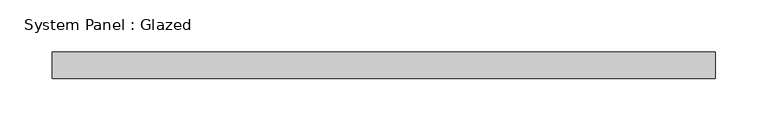
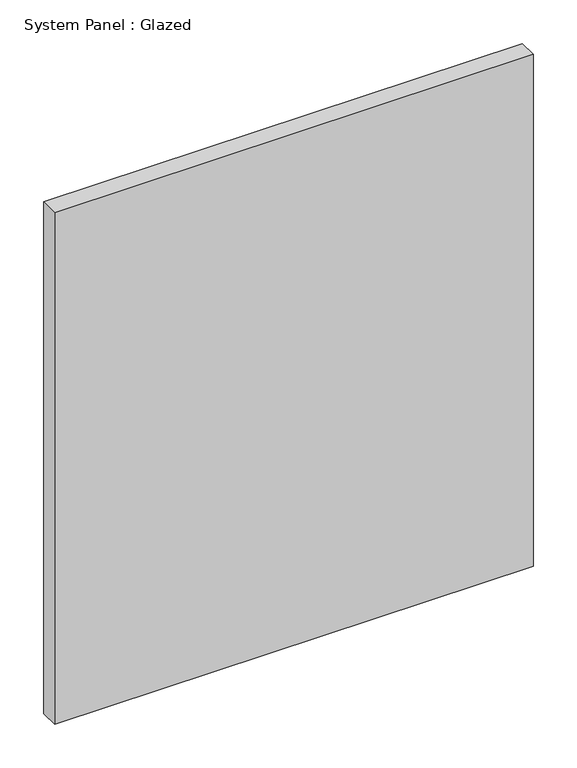
"""IFC4 building model written with IfcOpenShell, lengths in millimetres: plate geometry, System Panel : Glazed."""

from ifc_helpers import new_model, si_unit, origin, origin_with_axes, place, context, project, spatial, polyline, outline, extrude, source, transform, mapped, element, save


def system_panel_glazed_d7e326c9(model_context):
    return source(origin(), model_context, "Body", "SweptSolid", [
        extrude(outline(polyline([(317.5, 19.05), (-317.5, 19.05), (-317.5, 44.45), (317.5, 44.45), (317.5, 19.05)])), origin_with_axes(), (0.0, 0.0, 1.0), 717.55),
    ])


if __name__ == "__main__":
    model = new_model("IFC4")
    model_context = context("Model", 3, world=origin())
    ifc_project = project(units=[si_unit("LENGTHUNIT", "METRE", prefix="MILLI")], contexts=[model_context])
    site = spatial("IfcSite", under=ifc_project)
    building = spatial("IfcBuilding", under=site)
    placement = place(None, origin())
    system_panel_glazed_shape = system_panel_glazed_d7e326c9(model_context)
    element("IfcPlate", 1, ObjectType="System Panel : Glazed", at=placement, inside=building, context=model_context, shape_type="MappedRepresentation", body=[
        mapped(system_panel_glazed_shape, transform((0.0, 0.0, 0.0), x_axis=(1.0, 0.0, 0.0), y_axis=(0.0, 1.0, 0.0), z_axis=(0.0, 0.0, 1.0))),
    ])
    save(model, "model.ifc")

# Revit data of these elements
# Type "System Panel : Glazed"
#   Construction Type Id = "GSP4R"
#   Analytic Construction = "1/8 in Pilkington single glazing"
#   Visual Light Transmittance = 0.9
#   Solar Heat Gain Coefficient = 0.86
#   Heat Transfer Coefficient (U) = 1.18115 BTU/(h·ft²·°F)
#   Define Thermal Properties by = 1
# Element 1 (IfcPlate, "System Panel : Glazed")
#   Materials on its faces: "Glass"
# Materials
#   "Glass": class "Glass", colour RGB 0 128 192, transparency 0.75, Description = "Soda Lime Glass", Cost = 0
